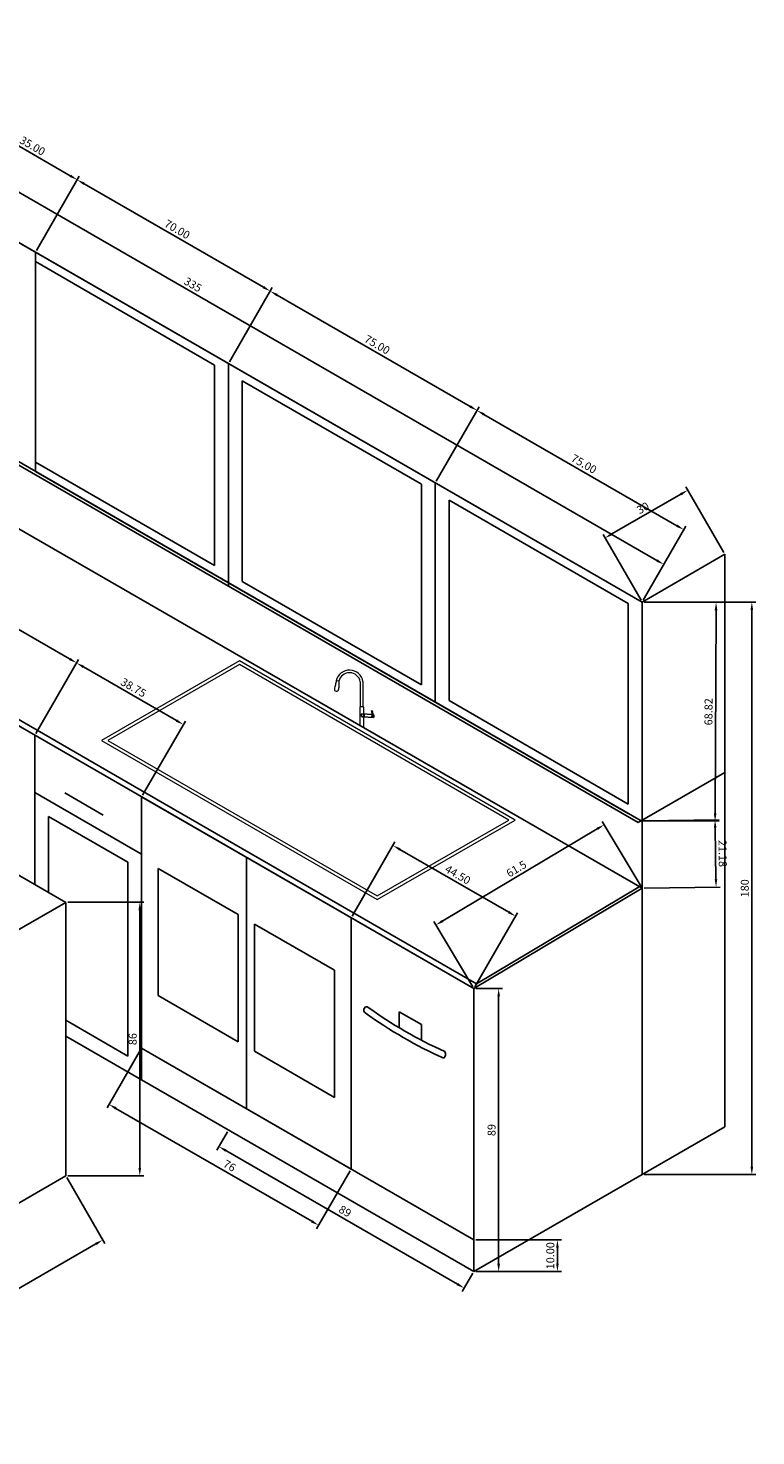
# Model space of a CAD drawing. Units: centimetres. Extents: x 21667 to 22807, y 15845 to 16565.
# Tile 2 of 4: x 21924 to 22153, y 15845 to 16287. Entities that reach past the tile are written whole.
import ezdxf

# ---------------------------------------------------------------- set-up
doc = ezdxf.new("R2010")
doc.units = ezdxf.units.CM
for name, color, linetype, lineweight in [('A-ANNO-DIMS', 2, 'Continuous', 18), ('A-ANNO-NPLT', 8, 'Continuous', 13), ('A-FLOR-FIXT', 4, 'Continuous', 18), ('A-FURN-CASE', 7, 'Continuous', 25)]:
    doc.layers.add(name, color=color, linetype=linetype, lineweight=lineweight)
doc.styles.get("Standard").update_dxf_attribs({"font": 'arial.ttf'})
doc.dimstyles.new('ISO-25', dxfattribs={"dimtxt": 2.5, "dimasz": 2.5, "dimexe": 1.25, "dimexo": 0.625, "dimtad": 1, "dimtxsty": 'Standard', "dimcen": 2.5, "dimadec": 0, "dimazin": 0, "dimtfac": 1, "dimtmove": 0, "dimatfit": 3, "dimfxl": 1, "dimarcsym": 0})

# ---------------------------------------------------------------- blocks, each defined once
blk = doc.blocks.new('*D1')
at = {"layer": 'A-ANNO-DIMS', "color": 0, "lineweight": -2, "transparency": 16777216}
for p, q in [((21986.67, 15940.31), (21983.36, 15934.57)), ((22058.89, 15892.41), (21986.15, 15934.41)), ((22063.74, 15895.81), (22060.43, 15890.07))]:
    blk.add_line(p, q, dxfattribs=at)
at = {"layer": 'A-ANNO-DIMS', "color": 0, "transparency": 16777216}
for points in [[(21986.35, 15934.77), (21985.94, 15934.05), (21983.98, 15935.66)], [(22059.1, 15892.77), (22058.68, 15892.05), (22061.06, 15891.16)]]:
    blk.add_solid(points, dxfattribs=at)
at = {"layer": 'Defpoints', "color": 0, "transparency": 16777216}
for p in [(21986.98, 15940.85), (21983.98, 15935.66), (22064.05, 15896.35)]:
    blk.add_point(p, dxfattribs=at)
at = {"layer": 'A-ANNO-DIMS', "color": 0, "transparency": 16777216, "insert": (22023.47, 15915.05), "char_height": 2.5, "attachment_point": 5, "rotation": 330}
blk.add_mtext('89', dxfattribs=at)
blk = doc.blocks.new('*D2')
at = {"layer": 'A-ANNO-DIMS', "color": 0, "lineweight": -2, "transparency": 16777216}
for p, q in [((22064.68, 15985.35), (22073.1, 15985.35)), ((22071.85, 15898.85), (22071.85, 15982.85)), ((22064.68, 15896.35), (22073.1, 15896.35))]:
    blk.add_line(p, q, dxfattribs=at)
at = {"layer": 'A-ANNO-DIMS', "color": 0, "transparency": 16777216}
for points in [[(22071.44, 15982.85), (22072.27, 15982.85), (22071.85, 15985.35)], [(22071.44, 15898.85), (22072.27, 15898.85), (22071.85, 15896.35)]]:
    blk.add_solid(points, dxfattribs=at)
at = {"layer": 'Defpoints', "color": 0, "transparency": 16777216}
for p in [(22064.05, 15985.35), (22071.85, 15985.35), (22064.05, 15896.35)]:
    blk.add_point(p, dxfattribs=at)
at = {"layer": 'A-ANNO-DIMS', "color": 0, "transparency": 16777216, "insert": (22069.95, 15940.85), "char_height": 2.5, "attachment_point": 5, "rotation": 90}
blk.add_mtext('89', dxfattribs=at)
blk = doc.blocks.new('*D3')
at = {"layer": 'A-ANNO-DIMS', "color": 0, "lineweight": -2, "transparency": 16777216}
for p, q in [((21959.39, 15966.06), (21948.86, 15947.83)), ((22013.14, 15912.16), (21951.65, 15947.66)), ((22025.2, 15928.06), (22014.68, 15909.83))]:
    blk.add_line(p, q, dxfattribs=at)
at = {"layer": 'A-ANNO-DIMS', "color": 0, "transparency": 16777216}
for points in [[(21951.86, 15948.02), (21951.44, 15947.3), (21949.49, 15948.91)], [(22013.35, 15912.52), (22012.93, 15911.8), (22015.31, 15910.91)]]:
    blk.add_solid(points, dxfattribs=at)
at = {"layer": 'Defpoints', "color": 0, "transparency": 16777216}
for p in [(21959.7, 15966.6), (21949.49, 15948.91), (22025.52, 15928.6)]:
    blk.add_point(p, dxfattribs=at)
at = {"layer": 'A-ANNO-DIMS', "color": 0, "transparency": 16777216, "insert": (21987.18, 15929.35), "char_height": 2.5, "attachment_point": 5, "rotation": 330}
blk.add_mtext('76', dxfattribs=at)
blk = doc.blocks.new('*D4')
at = {"layer": 'A-ANNO-DIMS', "color": 0, "lineweight": -2, "transparency": 16777216}
for p, q in [((21827.08, 16274.89), (21834.21, 16287.25)), ((21835.75, 16284.92), (22121.54, 16119.92)), ((22117.19, 16107.39), (22124.33, 16119.75))]:
    blk.add_line(p, q, dxfattribs=at)
at = {"layer": 'A-ANNO-DIMS', "color": 0, "transparency": 16777216}
for points in [[(21835.96, 16285.28), (21835.54, 16284.56), (21833.59, 16286.17)], [(22121.75, 16120.28), (22121.33, 16119.56), (22123.71, 16118.67)]]:
    blk.add_solid(points, dxfattribs=at)
at = {"layer": 'Defpoints', "color": 0, "transparency": 16777216}
for p in [(21826.76, 16274.35), (22123.71, 16118.67), (22116.88, 16106.85)]:
    blk.add_point(p, dxfattribs=at)
at = {"layer": 'A-ANNO-DIMS', "color": 0, "transparency": 16777216, "insert": (21975.66, 16206.34), "char_height": 2.5, "attachment_point": 5, "rotation": 330}
blk.add_mtext('335', dxfattribs=at)
blk = doc.blocks.new('*D5')
at = {"layer": 'A-ANNO-DIMS', "color": 0, "lineweight": -2, "transparency": 16777216}
for p, q in [((22117.51, 16106.85), (22152.62, 16106.85)), ((22151.37, 16104.35), (22151.37, 15929.35)), ((22117.51, 15926.85), (22152.62, 15926.85))]:
    blk.add_line(p, q, dxfattribs=at)
at = {"layer": 'A-ANNO-DIMS', "color": 0, "transparency": 16777216}
for points in [[(22150.95, 16104.35), (22151.78, 16104.35), (22151.37, 16106.85)], [(22150.95, 15929.35), (22151.78, 15929.35), (22151.37, 15926.85)]]:
    blk.add_solid(points, dxfattribs=at)
at = {"layer": 'Defpoints', "color": 0, "transparency": 16777216}
for p in [(22116.88, 16106.85), (22116.88, 15926.85), (22151.37, 15926.85)]:
    blk.add_point(p, dxfattribs=at)
at = {"layer": 'A-ANNO-DIMS', "color": 0, "transparency": 16777216, "insert": (22149.47, 16016.85), "char_height": 2.5, "attachment_point": 5, "rotation": 90}
blk.add_mtext('180', dxfattribs=at)
blk = doc.blocks.new('FAUCET')
for p, q in [((1.4, 14.57), (0.59, 14.75)), ((8.15, 14.4), (8.15, 6.62)), ((8.99, 14.47), (8.99, 6.62)), ((8.15, 6.62), (8.01, 6.3)), ((8.01, 6.3), (8.01, 0.66)), ((8.15, 6.62), (8.99, 6.62)), ((8.99, 6.62), (9.15, 6.35)), ((9.15, 6.35), (9.15, 0))]:
    blk.add_line(p, q)
for radius, start in [(4.28, 8.9589), (3.44, 9.9927)]:
    blk.add_arc((4.76, 13.81), radius, start, 167.251)
for points, knots in [([(0.59, 14.75), (0.5, 14.32), (0.32, 13.44), (0.11, 12.57), (0, 12.12)], [0, 0, 0, 0, 1.316127, 2.691834, 2.691834, 2.691834, 2.691834]), ([(1.4, 14.57), (1.41, 14.09), (1.41, 13.24), (1.35, 12.4), (1.32, 12.02)], [0, 0, 0, 0, 1.416831, 2.547877, 2.547877, 2.547877, 2.547877]), ([(0, 12.12), (0.01, 11.98), (0.03, 11.46), (1.13, 11.35), (1.28, 11.86), (1.32, 12.02)], [0, 0, 0, 0, 0.416688, 1.456431, 1.924702, 1.924702, 1.924702, 1.924702])]:
    blk.add_open_spline(points, degree=3, knots=knots)
blk = doc.blocks.new('*D16')
at = {"layer": 'A-ANNO-DIMS', "color": 0, "lineweight": -2, "transparency": 16777216}
for p, q in [((22117.51, 16106.85), (22141.38, 16106.74)), ((22140.12, 16104.25), (22139.84, 16040.42)), ((22117.2, 16038.02), (22141.07, 16037.92))]:
    blk.add_line(p, q, dxfattribs=at)
at = {"layer": 'A-ANNO-DIMS', "color": 0, "transparency": 16777216}
for points in [[(22139.7, 16104.25), (22140.54, 16104.24), (22140.13, 16106.75)], [(22139.42, 16040.43), (22140.25, 16040.42), (22139.82, 16037.92)]]:
    blk.add_solid(points, dxfattribs=at)
at = {"layer": 'Defpoints', "color": 0, "transparency": 16777216}
for p in [(22116.88, 16106.85), (22116.57, 16038.03), (22139.82, 16037.92)]:
    blk.add_point(p, dxfattribs=at)
at = {"layer": 'A-ANNO-DIMS', "color": 0, "transparency": 16777216, "insert": (22138.08, 16072.34), "char_height": 2.5, "attachment_point": 5, "rotation": 89.7433}
blk.add_mtext('68.82', dxfattribs=at)
blk = doc.blocks.new('*D17')
at = {"layer": 'A-ANNO-DIMS', "color": 0, "lineweight": -2, "transparency": 16777216}
for p, q in [((22107.42, 16128.23), (22129.07, 16140.73)), ((22142.55, 16122.39), (22130.61, 16143.07)), ((22116.57, 16107.39), (22104.63, 16128.07))]:
    blk.add_line(p, q, dxfattribs=at)
at = {"layer": 'A-ANNO-DIMS', "color": 0, "transparency": 16777216}
for points in [[(22128.86, 16141.1), (22129.28, 16140.37), (22131.24, 16141.98)], [(22107.21, 16128.6), (22107.63, 16127.87), (22105.26, 16126.98)]]:
    blk.add_solid(points, dxfattribs=at)
at = {"layer": 'Defpoints', "color": 0, "transparency": 16777216}
for p in [(22131.24, 16141.98), (22142.86, 16121.85), (22116.88, 16106.85)]:
    blk.add_point(p, dxfattribs=at)
at = {"layer": 'A-ANNO-DIMS', "color": 0, "transparency": 16777216, "insert": (22117.3, 16136.13), "char_height": 2.5, "attachment_point": 5, "rotation": 30}
blk.add_mtext('30', dxfattribs=at)
blk = doc.blocks.new('*D18')
at = {"layer": 'A-ANNO-DIMS', "color": 0, "lineweight": -2, "transparency": 16777216}
for p, q in [((22117.2, 16038.04), (22141.07, 16038.38)), ((22139.86, 16035.87), (22140.09, 16019.69)), ((22117.51, 16016.86), (22141.38, 16017.21))]:
    blk.add_line(p, q, dxfattribs=at)
at = {"layer": 'A-ANNO-DIMS', "color": 0, "transparency": 16777216}
for points in [[(22140.27, 16035.87), (22139.44, 16035.86), (22139.82, 16038.37)], [(22140.51, 16019.69), (22139.68, 16019.68), (22140.13, 16017.19)]]:
    blk.add_solid(points, dxfattribs=at)
at = {"layer": 'Defpoints', "color": 0, "transparency": 16777216}
for p in [(22116.57, 16038.03), (22116.88, 16016.85), (22140.13, 16017.19)]:
    blk.add_point(p, dxfattribs=at)
at = {"layer": 'A-ANNO-DIMS', "color": 0, "transparency": 16777216, "insert": (22141.88, 16027.8), "char_height": 2.5, "attachment_point": 5, "rotation": 270.8342}
blk.add_mtext('21.18', dxfattribs=at)
blk = doc.blocks.new('*D19')
at = {"layer": 'A-ANNO-DIMS', "color": 0, "lineweight": -2, "transparency": 16777216}
for p, q in [((22116.56, 16017.39), (22104.33, 16037.89)), ((22054.29, 16006.6), (22102.83, 16035.54)), ((22063.73, 15985.89), (22051.51, 16006.39))]:
    blk.add_line(p, q, dxfattribs=at)
at = {"layer": 'A-ANNO-DIMS', "color": 0, "transparency": 16777216}
for points in [[(22102.61, 16035.9), (22103.04, 16035.18), (22104.98, 16036.82)], [(22054.08, 16006.96), (22054.51, 16006.24), (22052.15, 16005.32)]]:
    blk.add_solid(points, dxfattribs=at)
at = {"layer": 'Defpoints', "color": 0, "transparency": 16777216}
for p in [(22104.98, 16036.82), (22116.88, 16016.85), (22064.05, 15985.35)]:
    blk.add_point(p, dxfattribs=at)
at = {"layer": 'A-ANNO-DIMS', "color": 0, "transparency": 16777216, "insert": (22077.59, 16022.7), "char_height": 2.5, "attachment_point": 5, "rotation": 30.8068}
blk.add_mtext('61.5', dxfattribs=at)
blk = doc.blocks.new('*D21')
at = {"layer": 'A-ANNO-DIMS', "color": 0, "lineweight": -2, "transparency": 16777216}
for p, q in [((21936.2, 15925.9), (21948.13, 15905.22)), ((21945.34, 15905.05), (21844.88, 15847.05)), ((21831.41, 15865.4), (21843.34, 15844.72))]:
    blk.add_line(p, q, dxfattribs=at)
at = {"layer": 'A-ANNO-DIMS', "color": 0, "transparency": 16777216}
for points in [[(21945.13, 15905.41), (21945.55, 15904.69), (21947.51, 15906.3)], [(21844.68, 15847.41), (21845.09, 15846.69), (21842.72, 15845.8)]]:
    blk.add_solid(points, dxfattribs=at)
at = {"layer": 'Defpoints', "color": 0, "transparency": 16777216}
for p in [(21935.88, 15926.44), (21831.09, 15865.94), (21842.72, 15845.8)]:
    blk.add_point(p, dxfattribs=at)
at = {"layer": 'A-ANNO-DIMS', "color": 0, "transparency": 16777216, "insert": (21894.17, 15877.68), "char_height": 2.5, "attachment_point": 5, "rotation": 30}
blk.add_mtext('121', dxfattribs=at)
blk = doc.blocks.new('*D22')
at = {"layer": 'A-ANNO-DIMS', "color": 0, "lineweight": -2, "transparency": 16777216}
for p, q in [((21936.51, 16012.44), (21960.38, 16012.44)), ((21959.13, 16009.94), (21959.13, 15928.94)), ((21936.51, 15926.44), (21960.38, 15926.44))]:
    blk.add_line(p, q, dxfattribs=at)
at = {"layer": 'A-ANNO-DIMS', "color": 0, "transparency": 16777216}
for points in [[(21958.72, 16009.94), (21959.55, 16009.94), (21959.13, 16012.44)], [(21958.72, 15928.94), (21959.55, 15928.94), (21959.13, 15926.44)]]:
    blk.add_solid(points, dxfattribs=at)
at = {"layer": 'Defpoints', "color": 0, "transparency": 16777216}
for p in [(21935.88, 16012.44), (21935.88, 15926.44), (21959.13, 15926.44)]:
    blk.add_point(p, dxfattribs=at)
at = {"layer": 'A-ANNO-DIMS', "color": 0, "transparency": 16777216, "insert": (21957.23, 15969.44), "char_height": 2.5, "attachment_point": 5, "rotation": 90}
blk.add_mtext('86', dxfattribs=at)
blk = doc.blocks.new('*D45')
at = {"layer": 'A-ANNO-DIMS', "color": 0, "lineweight": -2, "transparency": 16777216}
for p, q in [((21896.36, 16234.89), (21909.8, 16258.17)), ((21911.34, 16255.83), (21937.32, 16240.83)), ((21926.67, 16217.39), (21940.11, 16240.67))]:
    blk.add_line(p, q, dxfattribs=at)
at = {"layer": 'A-ANNO-DIMS', "color": 0, "transparency": 16777216}
for points in [[(21911.54, 16256.19), (21911.13, 16255.47), (21909.17, 16257.08)], [(21937.53, 16241.19), (21937.11, 16240.47), (21939.48, 16239.58)]]:
    blk.add_solid(points, dxfattribs=at)
at = {"layer": 'Defpoints', "color": 0, "transparency": 16777216}
for p in [(21939.48, 16239.58), (21896.05, 16234.35), (21926.36, 16216.85)]:
    blk.add_point(p, dxfattribs=at)
at = {"layer": 'A-ANNO-DIMS', "color": 0, "transparency": 16777216, "insert": (21925.28, 16249.98), "char_height": 2.5, "attachment_point": 5, "rotation": 330}
blk.add_mtext('35.00', dxfattribs=at)
blk = doc.blocks.new('*D46')
at = {"layer": 'A-ANNO-DIMS', "color": 0, "lineweight": -2, "transparency": 16777216}
for p, q in [((21926.67, 16217.39), (21940.11, 16240.67)), ((21941.65, 16238.33), (21997.94, 16205.83)), ((21987.29, 16182.39), (22000.73, 16205.67))]:
    blk.add_line(p, q, dxfattribs=at)
at = {"layer": 'A-ANNO-DIMS', "color": 0, "transparency": 16777216}
for points in [[(21941.86, 16238.69), (21941.44, 16237.97), (21939.48, 16239.58)], [(21998.15, 16206.19), (21997.73, 16205.47), (22000.1, 16204.58)]]:
    blk.add_solid(points, dxfattribs=at)
at = {"layer": 'Defpoints', "color": 0, "transparency": 16777216}
for p in [(21926.36, 16216.85), (22000.1, 16204.58), (21986.98, 16181.85)]:
    blk.add_point(p, dxfattribs=at)
at = {"layer": 'A-ANNO-DIMS', "color": 0, "transparency": 16777216, "insert": (21970.74, 16223.73), "char_height": 2.5, "attachment_point": 5, "rotation": 330}
blk.add_mtext('70.00', dxfattribs=at)
blk = doc.blocks.new('*D47')
at = {"layer": 'A-ANNO-DIMS', "color": 0, "lineweight": -2, "transparency": 16777216}
for p, q in [((21987.29, 16182.39), (22000.73, 16205.67)), ((22002.27, 16203.33), (22062.89, 16168.33)), ((22052.24, 16144.89), (22065.68, 16168.17))]:
    blk.add_line(p, q, dxfattribs=at)
at = {"layer": 'A-ANNO-DIMS', "color": 0, "transparency": 16777216}
for points in [[(22002.48, 16203.69), (22002.06, 16202.97), (22000.1, 16204.58)], [(22063.1, 16168.69), (22062.68, 16167.97), (22065.06, 16167.08)]]:
    blk.add_solid(points, dxfattribs=at)
at = {"layer": 'Defpoints', "color": 0, "transparency": 16777216}
for p in [(21986.98, 16181.85), (22065.06, 16167.08), (22051.93, 16144.35)]:
    blk.add_point(p, dxfattribs=at)
at = {"layer": 'A-ANNO-DIMS', "color": 0, "transparency": 16777216, "insert": (22033.53, 16187.48), "char_height": 2.5, "attachment_point": 5, "rotation": 330}
blk.add_mtext('75.00', dxfattribs=at)
blk = doc.blocks.new('*D48')
at = {"layer": 'A-ANNO-DIMS', "color": 0, "lineweight": -2, "transparency": 16777216}
for p, q in [((22052.24, 16144.89), (22065.68, 16168.17)), ((22067.22, 16165.83), (22127.84, 16130.83)), ((22117.19, 16107.39), (22130.63, 16130.67))]:
    blk.add_line(p, q, dxfattribs=at)
at = {"layer": 'A-ANNO-DIMS', "color": 0, "transparency": 16777216}
for points in [[(22067.43, 16166.19), (22067.01, 16165.47), (22065.06, 16167.08)], [(22128.05, 16131.19), (22127.63, 16130.47), (22130.01, 16129.58)]]:
    blk.add_solid(points, dxfattribs=at)
at = {"layer": 'Defpoints', "color": 0, "transparency": 16777216}
for p in [(22051.93, 16144.35), (22130.01, 16129.58), (22116.88, 16106.85)]:
    blk.add_point(p, dxfattribs=at)
at = {"layer": 'A-ANNO-DIMS', "color": 0, "transparency": 16777216, "insert": (22098.48, 16149.98), "char_height": 2.5, "attachment_point": 5, "rotation": 330}
blk.add_mtext('75.00', dxfattribs=at)
blk = doc.blocks.new('*D50')
at = {"layer": 'A-ANNO-DIMS', "color": 0, "lineweight": -2, "transparency": 16777216}
for p, q in [((21860.63, 16103.52), (21874.07, 16126.79)), ((21875.61, 16124.46), (21937.1, 16088.96)), ((21926.45, 16065.52), (21939.89, 16088.79))]:
    blk.add_line(p, q, dxfattribs=at)
at = {"layer": 'A-ANNO-DIMS', "color": 0, "transparency": 16777216}
for points in [[(21875.82, 16124.82), (21875.4, 16124.1), (21873.45, 16125.71)], [(21937.31, 16089.32), (21936.89, 16088.6), (21939.27, 16087.71)]]:
    blk.add_solid(points, dxfattribs=at)
at = {"layer": 'Defpoints', "color": 0, "transparency": 16777216}
for p in [(21860.32, 16102.97), (21939.27, 16087.71), (21926.14, 16064.97)]:
    blk.add_point(p, dxfattribs=at)
at = {"layer": 'A-ANNO-DIMS', "color": 0, "transparency": 16777216, "insert": (21907.31, 16108.35), "char_height": 2.5, "attachment_point": 5, "rotation": 330}
blk.add_mtext('76.00', dxfattribs=at)
blk = doc.blocks.new('*D51')
at = {"layer": 'A-ANNO-DIMS', "color": 0, "lineweight": -2, "transparency": 16777216}
for p, q in [((21926.45, 16065.52), (21939.89, 16088.79)), ((21941.43, 16086.46), (21970.66, 16069.58)), ((21960.01, 16046.14), (21973.45, 16069.42))]:
    blk.add_line(p, q, dxfattribs=at)
at = {"layer": 'A-ANNO-DIMS', "color": 0, "transparency": 16777216}
for points in [[(21941.64, 16086.82), (21941.22, 16086.1), (21939.27, 16087.71)], [(21970.87, 16069.94), (21970.45, 16069.22), (21972.82, 16068.33)]]:
    blk.add_solid(points, dxfattribs=at)
at = {"layer": 'Defpoints', "color": 0, "transparency": 16777216}
for p in [(21972.82, 16068.33), (21926.14, 16064.97), (21959.7, 16045.6)]:
    blk.add_point(p, dxfattribs=at)
at = {"layer": 'A-ANNO-DIMS', "color": 0, "transparency": 16777216, "insert": (21957, 16079.67), "char_height": 2.5, "attachment_point": 5, "rotation": 330}
blk.add_mtext('38.75', dxfattribs=at)
blk = doc.blocks.new('*D52')
at = {"layer": 'A-ANNO-DIMS', "color": 0, "lineweight": -2, "transparency": 16777216}
for p, q in [((22025.83, 16008.14), (22039.27, 16031.42)), ((22040.81, 16029.08), (22075.01, 16009.33)), ((22064.37, 15985.89), (22077.8, 16009.17))]:
    blk.add_line(p, q, dxfattribs=at)
at = {"layer": 'A-ANNO-DIMS', "color": 0, "transparency": 16777216}
for points in [[(22041.02, 16029.44), (22040.6, 16028.72), (22038.64, 16030.33)], [(22075.22, 16009.69), (22074.81, 16008.97), (22077.18, 16008.08)]]:
    blk.add_solid(points, dxfattribs=at)
at = {"layer": 'Defpoints', "color": 0, "transparency": 16777216}
for p in [(22025.52, 16007.6), (22077.18, 16008.08), (22064.05, 15985.35)]:
    blk.add_point(p, dxfattribs=at)
at = {"layer": 'A-ANNO-DIMS', "color": 0, "transparency": 16777216, "insert": (22058.86, 16020.85), "char_height": 2.5, "attachment_point": 5, "rotation": 330}
blk.add_mtext('44.50', dxfattribs=at)
blk = doc.blocks.new('*D53')
at = {"layer": 'A-ANNO-DIMS', "color": 0, "lineweight": -2, "transparency": 16777216}
for p, q in [((22064.68, 15906.35), (22091.55, 15906.35)), ((22090.3, 15903.85), (22090.3, 15898.85)), ((22064.68, 15896.35), (22091.55, 15896.35))]:
    blk.add_line(p, q, dxfattribs=at)
at = {"layer": 'A-ANNO-DIMS', "color": 0, "transparency": 16777216}
for points in [[(22089.89, 15903.85), (22090.72, 15903.85), (22090.3, 15906.35)], [(22089.89, 15898.85), (22090.72, 15898.85), (22090.3, 15896.35)]]:
    blk.add_solid(points, dxfattribs=at)
at = {"layer": 'Defpoints', "color": 0, "transparency": 16777216}
for p in [(22064.05, 15906.35), (22064.05, 15896.35), (22090.3, 15896.35)]:
    blk.add_point(p, dxfattribs=at)
at = {"layer": 'A-ANNO-DIMS', "color": 0, "transparency": 16777216, "insert": (22088.4, 15901.35), "char_height": 2.5, "attachment_point": 5, "rotation": 90}
blk.add_mtext('10.00', dxfattribs=at)

msp = doc.modelspace()

# ---------------------------------------------------------------- linework, layer by layer
at = {"layer": 'A-ANNO-NPLT'}
for p in [(21986.9786, 16181.8494), (22051.9305, 16144.3494)]:
    msp.add_point(p, dxfattribs=at)
at = {"layer": 'A-FLOR-FIXT'}
for points in [[(22077.0424, 16038.3188), (21990.4399, 16088.3188), (21947.1386, 16063.3188), (22033.7412, 16013.3188)], [(22075.0424, 16038.3188), (21990.4399, 16087.1641), (21949.1386, 16063.3188), (22033.7412, 16014.4735)]]:
    msp.add_lwpolyline(points, close=True, dxfattribs=at)
at = {"layer": 'A-FURN-CASE'}
for p, q in [((22116.8824, 16106.8494), (21826.7639, 16274.3494)), ((21922.0267, 16219.3494), (22116.8824, 16106.8494)), ((21926.3568, 16216.8494), (21926.3568, 16147.8494)), ((21926.3568, 16213.8494), (21982.6485, 16181.3494)), ((21826.7639, 16205.3494), (22116.574, 16038.0275)), ((21826.7639, 16204.3494), (22115.708, 16037.5275)), ((22116.8824, 16016.8494), (21826.7639, 16184.3494)), ((21982.6485, 16181.3494), (21982.6485, 16118.3494)), ((21986.9786, 16181.8494), (21986.9786, 16111.8494)), ((21991.3087, 16176.3494), (21991.3087, 16113.3494)), ((21991.3087, 16176.3494), (22047.6004, 16143.8494)), ((21926.3568, 16150.8494), (21982.6485, 16118.3494)), ((21926.3568, 16147.8494), (22112.5523, 16040.3494)), ((22047.6004, 16143.8494), (22047.6004, 16080.8494)), ((22051.9305, 16144.3494), (22051.9305, 16075.3494)), ((22056.2606, 16138.8494), (22056.2606, 16075.8494)), ((22056.2606, 16138.8494), (22112.5523, 16106.3494)), ((22064.0549, 15985.3494), (21825.8979, 16122.8494)), ((21961.4308, 16046.5994), (21826.0621, 16124.7546)), ((22116.8824, 16106.8494), (22142.8632, 16121.8494)), ((22142.8632, 15941.8494), (22142.8632, 16121.8494)), ((21991.3087, 16113.3494), (22047.6004, 16080.8494)), ((22112.5523, 16043.3494), (22112.5523, 16106.3494)), ((22116.8824, 15926.8494), (22116.8824, 16106.8494)), ((21935.8831, 16012.438), (21831.094, 16072.938)), ((22056.2606, 16075.8494), (22112.5523, 16043.3494)), ((22028.9161, 16071.7173), (22032.337, 16071.5137)), ((22029.1092, 16070.7317), (22032.5278, 16070.5282)), ((21926.1403, 16064.9744), (21926.1403, 16018.063)), ((22115.708, 16037.5275), (22142.8632, 16053.2055)), ((21959.6988, 16027.5819), (21926.1403, 16046.9569)), ((21935.5657, 16046.8351), (21947.6728, 16039.845)), ((21961.4308, 16046.5994), (22064.8929, 15986.8656)), ((21959.6988, 16045.5994), (22064.0549, 15985.3494)), ((21959.6988, 15956.5994), (21959.6988, 16045.5994)), ((21930.4704, 16039.4569), (21930.4704, 16015.563)), ((21955.3687, 16025.0819), (21930.4704, 16039.4569)), ((21955.3687, 15964.0994), (21955.3687, 16025.0819)), ((21992.6078, 15947.5994), (21992.6078, 16026.5994)), ((21990.0097, 16008.5994), (21964.8949, 16023.0994)), ((21964.8949, 16023.0994), (21964.8949, 15983.0994)), ((21992.6078, 15950.5994), (21992.6078, 16023.5994)), ((22064.0549, 15985.3494), (22116.8824, 16016.8494)), ((22064.8929, 15986.8656), (22116.0164, 16017.3494)), ((21831.094, 15951.938), (21935.8831, 16012.438)), ((21935.8831, 16012.438), (21935.8831, 15926.438)), ((21990.0097, 15968.5994), (21990.0097, 16008.5994)), ((22025.5167, 15928.5994), (22025.5167, 16007.5994)), ((21995.2058, 15965.5994), (21995.2058, 16005.5994)), ((22020.3206, 15991.0994), (21995.2058, 16005.5994)), ((22020.3206, 15951.0994), (22020.3206, 15991.0994)), ((22064.0549, 15896.3494), (22064.0549, 15985.3494)), ((22065.759, 15986.3656), (22065.7869, 15986.3494)), ((21990.0097, 15968.5994), (21964.8949, 15983.0994)), ((21955.3687, 15964.0994), (21935.8831, 15975.3494)), ((22040.555, 15973.0205), (22040.555, 15978.049)), ((22040.555, 15978.049), (22047.569, 15973.9995)), ((22047.569, 15973.9995), (22047.569, 15969.0888)), ((21959.6988, 15956.5994), (21935.8831, 15970.3494)), ((22064.0549, 15906.3494), (21959.6988, 15966.5994)), ((21959.6988, 15966.5994), (22025.5167, 15928.5994)), ((22020.3206, 15951.0994), (21995.2058, 15965.5994)), ((22064.0549, 15896.3494), (21959.6988, 15956.5994)), ((22116.8824, 15926.8494), (22142.8632, 15941.8494)), ((22116.8824, 15926.8494), (22064.0549, 15896.3494)), ((21935.8831, 15926.438), (21831.094, 15865.938))]:
    msp.add_line(p, q, dxfattribs=at)
for centre, radius, start, end in [((22029.2756, 16071.276), 0.5692, 129.168141, 253.001145), ((22028.7428, 16071.1072), 0.8739, 332.759171, 41.722153), ((22032.0207, 16072.5605), 0.1083, 11.472802, 160.933429), ((22029.7587, 16071.5918), 2.3816, 343.073014, 24.934412), ((22032.1497, 16071.0171), 0.1636, 226.514294, 305.891937), ((22029.9671, 16071.578), 2.3816, 343.073014, 24.934412), ((22032.0839, 16070.9535), 0.6148, 316.230119, 65.688838), ((22030.5247, 15978.5571), 1.0661, 88.202964, 234.688572), ((22113.4558, 16093.8934), 143.1225, 234.285483, 245.709216), ((22111.3286, 16091.0553), 137.6267, 234.06401, 245.822186), ((22053.3673, 15964.7153), 1.7706, 313.751182, 26.574086)]:
    msp.add_arc(centre, radius, start, end, dxfattribs=at)

# ---------------------------------------------------------------- block references
at = {"layer": 'A-FLOR-FIXT'}
msp.add_blockref('FAUCET', (22020.249, 16067.36), dxfattribs=at)

# ---------------------------------------------------------------- dimensions: what is measured, and where the dimension line sits
at = {"layer": 'A-ANNO-DIMS'}
for base, p1, p2, angle, picture, middle in [((22123.7059, 16118.668), (21826.7639, 16274.3494), (22116.8824, 16106.8494), 330, '*D4', (21974.7095, 16204.6911)), ((21949.4881, 15948.914), (22025.5167, 15928.5994), (21959.6988, 15966.5994), 150, '*D3', (21986.2303, 15927.7009))]:
    dim = msp.add_linear_dim(base=base, p1=p1, p2=p2, angle=angle, dimstyle='ISO-25', override={"dimclrd": 0, "dimclre": 0, "dimclrt": 0}, dxfattribs=at)
    dim.commit()
    dim.dimension.update_dxf_attribs({"geometry": picture, "text_midpoint": middle, "dimtype": 161})
for base, p1, p2, angle, override, picture, middle in [((21939.4818, 16239.5826), (21896.0459, 16234.3494), (21926.3568, 16216.8494), 330, {"dimdec": 2, "dimlfac": 1, "dimrnd": 0, "dimzin": 0, "dimdsep": 46, "dimlunit": 2}, '*D45', (21925.2775, 16249.98)), ((22000.1036, 16204.5826), (21926.3568, 16216.8494), (21986.9786, 16181.8494), 330, {"dimdec": 2, "dimlfac": 1, "dimrnd": 0, "dimzin": 0, "dimdsep": 46, "dimlunit": 2}, '*D46', (21970.7434, 16223.7293)), ((22065.0555, 16167.0826), (21986.9786, 16181.8494), (22051.9305, 16144.3494), 330, {"dimdec": 2, "dimlfac": 1, "dimrnd": 0, "dimzin": 0, "dimdsep": 46, "dimlunit": 2}, '*D47', (22033.5303, 16187.4793)), ((22130.0074, 16129.5826), (22051.9305, 16144.3494), (22116.8824, 16106.8494), 330, {"dimdec": 2, "dimlfac": 1, "dimrnd": 0, "dimzin": 0, "dimdsep": 46, "dimlunit": 2}, '*D48', (22098.4822, 16149.9793)), ((22131.2382, 16141.9845), (22116.8824, 16106.8494), (22142.8632, 16121.8494), 30, {"dimdec": 0, "dimlfac": 1, "dimrnd": 0, "dimzin": 0, "dimdsep": 46, "dimlunit": 2}, '*D17', (22117.2966, 16136.1319)), ((21939.2653, 16087.7076), (21860.3224, 16102.9744), (21926.1403, 16064.9744), 330, {"dimdec": 2, "dimlfac": 1, "dimrnd": 0, "dimzin": 0, "dimdsep": 46, "dimlunit": 2}, '*D50', (21907.3071, 16108.3543)), ((22139.8238, 16037.9233), (22116.8824, 16106.8494), (22116.574, 16038.0275), 269.743286, {"dimdec": 2, "dimlfac": 1, "dimrnd": 0, "dimzin": 0, "dimdsep": 46, "dimlunit": 2}, '*D16', (22138.0766, 16072.3428)), ((21972.8238, 16068.3326), (21926.1403, 16064.9744), (21959.6988, 16045.5994), 330, {"dimdec": 2, "dimlfac": 1, "dimrnd": 0, "dimzin": 0, "dimdsep": 46, "dimlunit": 2}, '*D51', (21956.9957, 16079.6675)), ((22104.975, 16036.8188), (22064.0549, 15985.3494), (22116.8824, 16016.8494), 30.806769, {"dimdec": 1, "dimlfac": 1, "dimrnd": 0, "dimzin": 0, "dimdsep": 46, "dimlunit": 2}, '*D19', (22077.5875, 16022.702)), ((22140.1299, 16017.1879), (22116.574, 16038.0275), (22116.8824, 16016.8494), 270.834188, {"dimdec": 2, "dimlfac": 1, "dimrnd": 0, "dimzin": 0, "dimdsep": 46, "dimlunit": 2}, '*D18', (22141.877, 16027.8046)), ((22077.1799, 16008.0826), (22025.5167, 16007.5994), (22064.0549, 15985.3494), 330, {"dimdec": 2, "dimlfac": 1, "dimrnd": 0, "dimzin": 0, "dimdsep": 46, "dimlunit": 2}, '*D52', (22058.8615, 16020.8543)), ((21959.1331, 15926.438), (21935.8831, 16012.438), (21935.8831, 15926.438), 270, {"dimdec": 0, "dimlfac": 1, "dimrnd": 0, "dimzin": 0, "dimdsep": 46, "dimlunit": 2}, '*D22', (21957.2317, 15969.438)), ((21842.719, 15845.8029), (21935.8831, 15926.438), (21831.094, 15865.938), 210, {"dimdec": 0, "dimlfac": 1, "dimrnd": 0, "dimzin": 0, "dimdsep": 46, "dimlunit": 2}, '*D21', (21894.1735, 15877.6811)), ((22090.3049, 15896.3494), (22064.0549, 15906.3494), (22064.0549, 15896.3494), 270, {"dimdec": 2, "dimlfac": 1, "dimrnd": 0, "dimzin": 0, "dimdsep": 46, "dimlunit": 2}, '*D53', (22088.4034, 15901.3494))]:
    dim = msp.add_linear_dim(base=base, p1=p1, p2=p2, angle=angle, dimstyle='ISO-25', override=override, dxfattribs=at)
    dim.commit()
    dim.dimension.update_dxf_attribs({"geometry": picture, "text_midpoint": middle})
for p1, p2, distance, picture, middle in [((22116.8824, 16106.8494), (22116.8824, 15926.8494), 34.485, '*D5', (22149.466, 16016.8494)), ((22064.0549, 15896.3494), (22064.0549, 15985.3494), -7.7989, '*D2', (22069.9523, 15940.8494)), ((22064.0549, 15896.3494), (21986.9786, 15940.8494), 5.9961, '*D1', (22023.4694, 15915.0533))]:
    dim = msp.add_aligned_dim(p1=p1, p2=p2, distance=distance, dimstyle='ISO-25', override={"dimclrd": 0, "dimclre": 0, "dimclrt": 0}, dxfattribs=at)
    dim.commit()
    dim.dimension.update_dxf_attribs({"geometry": picture, "text_midpoint": middle})

doc.saveas('drawing.dxf')
